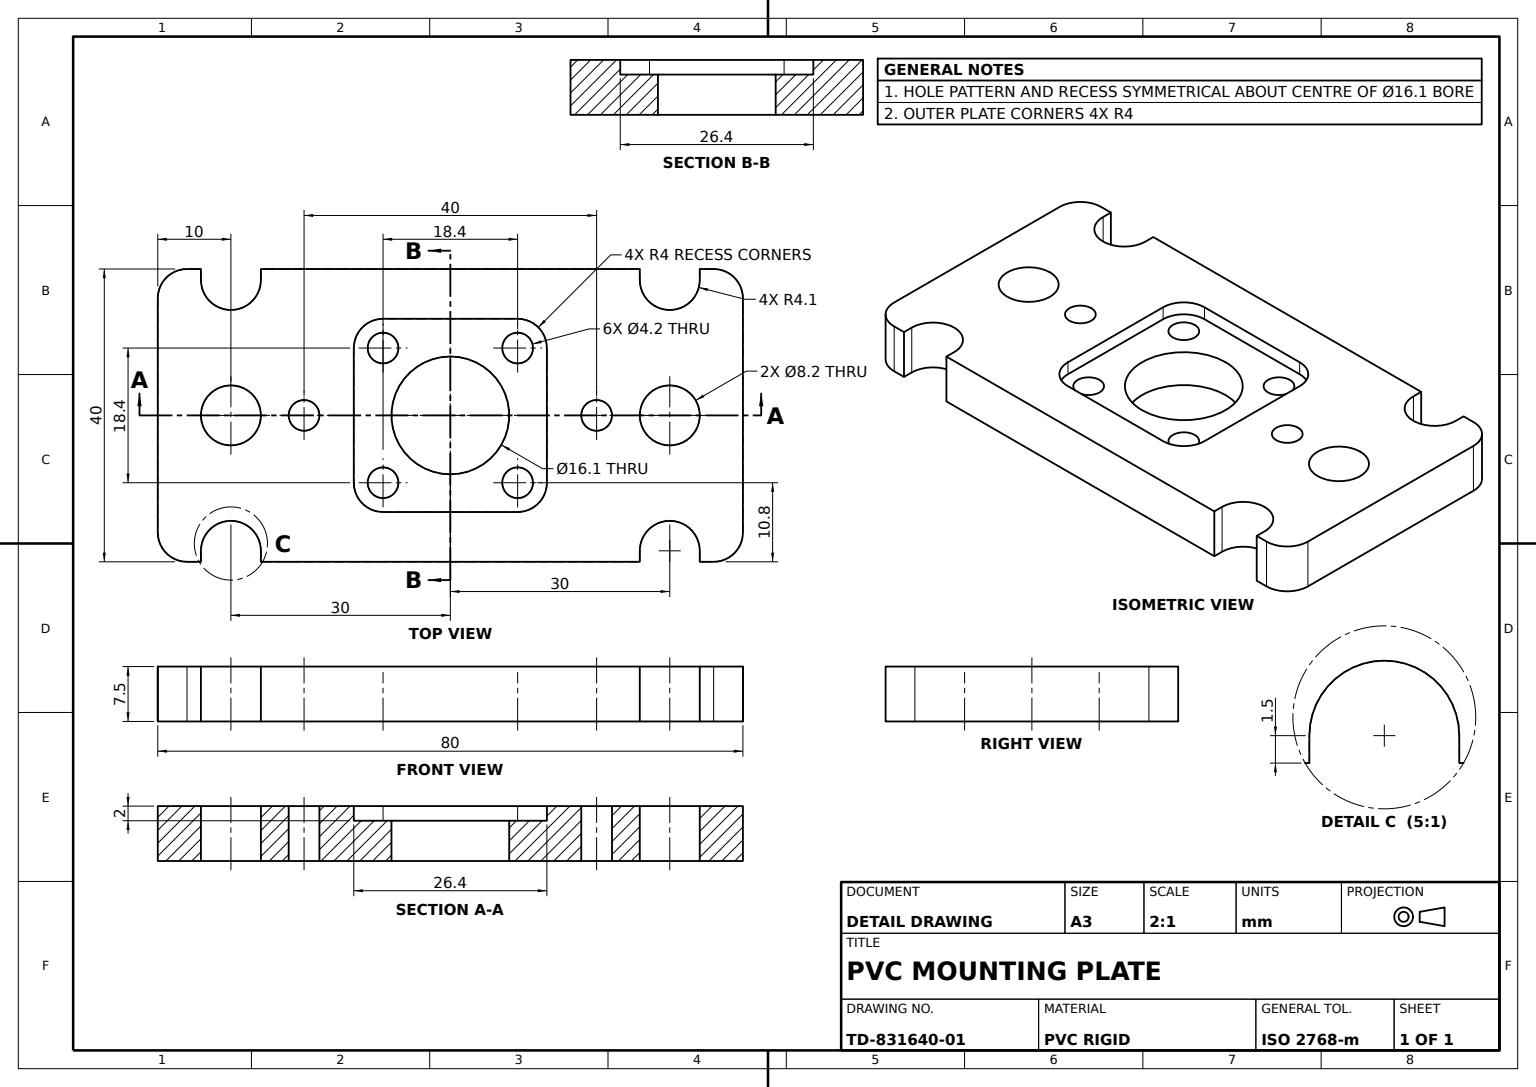
from build123d import *

# Parameters (mm, degrees)
BASE_PLATE_PROFILE_SKETCH_R               = 4.1
BASE_PLATE_PROFILE_SKETCH_R_2             = 2.1
BASE_PLATE_7_5MM_DEPTH                    = 7.5
CONNECTOR_RECESS_26_4MM_X_2MM_DEPTH       = 2
CONNECTOR_BORE_AND_SCREW_HOLES_REACH      = 47.058
CONNECTOR_BORE_AND_SCREW_HOLES_SKETCH_R   = 8.05
CONNECTOR_BORE_AND_SCREW_HOLES_SKETCH_R_2 = 2.1


with BuildPart() as part:
    # Base Plate Profile Sketch → Base Plate 7.5mm (new body)
    with BuildSketch(Plane(origin=(0, 0, 0), x_dir=(1, 0, 0), z_dir=(0, 1, 0))):
        with BuildLine():
            Line((-34.1, 20), (-34.1, 18.5))
            ThreePointArc((-34.1, 18.5), (-30, 14.4), (-25.9, 18.5))
            Line((-25.9, 18.5), (-25.9, 20))
            Line((-25.9, 20), (25.9, 20))
            Line((25.9, 20), (25.9, 18.5))
            ThreePointArc((25.9, 18.5), (30, 14.4), (34.1, 18.5))
            Line((34.1, 18.5), (34.1, 20))
            Line((34.1, 20), (36, 20))
            ThreePointArc((36, 20), (38.828427125, 18.828427125), (40, 16))
            Line((40, 16), (40, -16))
            ThreePointArc((40, -16), (38.828427125, -18.828427125), (36, -20))
            Line((36, -20), (34.1, -20))
            Line((34.1, -20), (34.1, -18.5))
            ThreePointArc((34.1, -18.5), (30, -14.4), (25.9, -18.5))
            Line((25.9, -18.5), (25.9, -20))
            Line((25.9, -20), (-25.9, -20))
            Line((-25.9, -20), (-25.9, -18.5))
            ThreePointArc((-25.9, -18.5), (-30, -14.4), (-34.1, -18.5))
            Line((-34.1, -18.5), (-34.1, -20))
            Line((-34.1, -20), (-36, -20))
            ThreePointArc((-36, -20), (-38.828427125, -18.828427125), (-40, -16))
            Line((-40, -16), (-40, 16))
            ThreePointArc((-40, 16), (-38.828427125, 18.828427125), (-36, 20))
            Line((-36, 20), (-34.1, 20))
        make_face()
        with Locations(Location((-30, 0, 0), (0, 0, 270))):
            Circle(BASE_PLATE_PROFILE_SKETCH_R, mode=Mode.SUBTRACT)
        with Locations(Location((30, 0, 0), (0, 0, 90))):
            Circle(BASE_PLATE_PROFILE_SKETCH_R, mode=Mode.SUBTRACT)
        with Locations(Location((-20, 0, 0), (0, 0, 270))):
            Circle(BASE_PLATE_PROFILE_SKETCH_R_2, mode=Mode.SUBTRACT)
        with Locations(Location((20, 0, 0), (0, 0, 90))):
            Circle(BASE_PLATE_PROFILE_SKETCH_R_2, mode=Mode.SUBTRACT)
    extrude(amount=BASE_PLATE_7_5MM_DEPTH)

    # Connector Recess Sketch → Connector Recess 26.4mm x 2mm (cut)
    with BuildSketch(Plane(origin=(0, 7.5, 0), x_dir=(1, 0, 0), z_dir=(0, 1, 0))):
        with BuildLine():
            Line((-9.2, -13.2), (9.2, -13.2))
            ThreePointArc((9.2, -13.2), (12.028427125, -12.028427125), (13.2, -9.2))
            Line((13.2, -9.2), (13.2, 9.2))
            ThreePointArc((13.2, 9.2), (12.028427125, 12.028427125), (9.2, 13.2))
            Line((9.2, 13.2), (-9.2, 13.2))
            ThreePointArc((-9.2, 13.2), (-12.028427125, 12.028427125), (-13.2, 9.2))
            Line((-13.2, 9.2), (-13.2, -9.2))
            ThreePointArc((-13.2, -9.2), (-12.028427125, -12.028427125), (-9.2, -13.2))
        make_face()
    extrude(amount=-CONNECTOR_RECESS_26_4MM_X_2MM_DEPTH, mode=Mode.SUBTRACT)

    # Connector Bore and Screw Holes Sketch → Connector Bore and Screw Holes (cut, up to next)
    with BuildSketch(Plane(origin=(0, 5.5, 0), x_dir=(1, 0, 0), z_dir=(0, 1, 0)), mode=Mode.PRIVATE) as connector_bore_and_screw_holes_sk1:
        with Locations(Location((0, 0, 0), (0, 0, 270))):
            Circle(CONNECTOR_BORE_AND_SCREW_HOLES_SKETCH_R)
    connector_bore_and_screw_holes_tool1 = extrude(connector_bore_and_screw_holes_sk1.sketch, amount=-CONNECTOR_BORE_AND_SCREW_HOLES_REACH, mode=Mode.PRIVATE) & part.part
    # Connector Bore and Screw Holes Sketch → Connector Bore and Screw Holes (cut, up to next)
    with BuildSketch(Plane(origin=(0, 5.5, 0), x_dir=(1, 0, 0), z_dir=(0, 1, 0)), mode=Mode.PRIVATE) as connector_bore_and_screw_holes_sk2:
        with Locations(Location((-9.2, 9.2, 0), (0, 0, 270))):
            Circle(CONNECTOR_BORE_AND_SCREW_HOLES_SKETCH_R_2)
    connector_bore_and_screw_holes_tool2 = extrude(connector_bore_and_screw_holes_sk2.sketch, amount=-CONNECTOR_BORE_AND_SCREW_HOLES_REACH, mode=Mode.PRIVATE) & part.part
    # Connector Bore and Screw Holes Sketch → Connector Bore and Screw Holes (cut, up to next)
    with BuildSketch(Plane(origin=(0, 5.5, 0), x_dir=(1, 0, 0), z_dir=(0, 1, 0)), mode=Mode.PRIVATE) as connector_bore_and_screw_holes_sk3:
        with Locations(Location((-9.2, -9.2, 0), (0, 0, 270))):
            Circle(CONNECTOR_BORE_AND_SCREW_HOLES_SKETCH_R_2)
    connector_bore_and_screw_holes_tool3 = extrude(connector_bore_and_screw_holes_sk3.sketch, amount=-CONNECTOR_BORE_AND_SCREW_HOLES_REACH, mode=Mode.PRIVATE) & part.part
    # Connector Bore and Screw Holes Sketch → Connector Bore and Screw Holes (cut, up to next)
    with BuildSketch(Plane(origin=(0, 5.5, 0), x_dir=(1, 0, 0), z_dir=(0, 1, 0)), mode=Mode.PRIVATE) as connector_bore_and_screw_holes_sk4:
        with Locations(Location((9.2, -9.2, 0), (0, 0, 270))):
            Circle(CONNECTOR_BORE_AND_SCREW_HOLES_SKETCH_R_2)
    connector_bore_and_screw_holes_tool4 = extrude(connector_bore_and_screw_holes_sk4.sketch, amount=-CONNECTOR_BORE_AND_SCREW_HOLES_REACH, mode=Mode.PRIVATE) & part.part
    # Connector Bore and Screw Holes Sketch → Connector Bore and Screw Holes (cut, up to next)
    with BuildSketch(Plane(origin=(0, 5.5, 0), x_dir=(1, 0, 0), z_dir=(0, 1, 0)), mode=Mode.PRIVATE) as connector_bore_and_screw_holes_sk5:
        with Locations(Location((9.2, 9.2, 0), (0, 0, 270))):
            Circle(CONNECTOR_BORE_AND_SCREW_HOLES_SKETCH_R_2)
    connector_bore_and_screw_holes_tool5 = extrude(connector_bore_and_screw_holes_sk5.sketch, amount=-CONNECTOR_BORE_AND_SCREW_HOLES_REACH, mode=Mode.PRIVATE) & part.part
    add(connector_bore_and_screw_holes_tool1.solids().sort_by_distance((0, 5.5, 0))[0], mode=Mode.SUBTRACT)
    add(connector_bore_and_screw_holes_tool2.solids().sort_by_distance((-9.2, 5.5, -9.2))[0], mode=Mode.SUBTRACT)
    add(connector_bore_and_screw_holes_tool3.solids().sort_by_distance((-9.2, 5.5, 9.2))[0], mode=Mode.SUBTRACT)
    add(connector_bore_and_screw_holes_tool4.solids().sort_by_distance((9.2, 5.5, 9.2))[0], mode=Mode.SUBTRACT)
    add(connector_bore_and_screw_holes_tool5.solids().sort_by_distance((9.2, 5.5, -9.2))[0], mode=Mode.SUBTRACT)


solid = part.part
